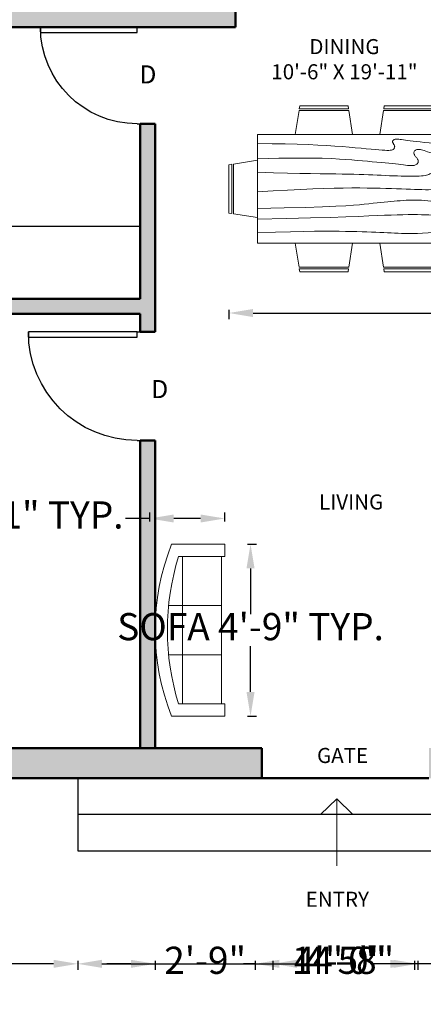
# Model space of a CAD drawing. Units: inches. Extents: x 2568 to 3190, y 746 to 1467.
# Tile 2 of 7: x 2767 to 2900, y 746 to 1073. Entities that reach past the tile are written whole.
import ezdxf

# ---------------------------------------------------------------- set-up
doc = ezdxf.new("R2010")
doc.units = ezdxf.units.IN
for name, color, linetype, lineweight in [('A-ANNO-DIMS', 2, 'Continuous', 18), ('A-ANNO-SYMB', 7, 'Continuous', 18), ('A-ANNO-TEXT', 7, 'Continuous', 18), ('A-AREA-IDEN', 7, 'Continuous', 25), ('A-DOOR', 3, 'Continuous', 25), ('A-FLOR-CASE', 8, 'Continuous', 25), ('A-FLOR-STRS', 7, 'Continuous', 25), ('A-FURN', 8, 'Continuous', 18), ('A-WALL', 7, 'Continuous', 50), ('A-WALL-PATT', 252, 'Continuous', 13)]:
    doc.layers.add(name, color=color, linetype=linetype, lineweight=lineweight)
doc.styles.get("Standard").update_dxf_attribs({"font": 'arial.ttf'})
doc.dimstyles.new('ISO-25', dxfattribs={"dimtxt": 9, "dimasz": 8, "dimexe": 2, "dimexo": 1, "dimtad": 0, "dimtih": 1, "dimtoh": 1, "dimdec": 1, "dimlunit": 3, "dimtxsty": 'Standard', "dimcen": 2.5, "dimclrd": 1, "dimclre": 3, "dimclrt": 6, "dimadec": 0, "dimazin": 0, "dimtfac": 1, "dimtdec": 1, "dimtmove": 0, "dimatfit": 3, "dimfxl": 1, "dimfxlon": 1, "dimarcsym": 0})

# ---------------------------------------------------------------- blocks, each defined once
blk = doc.blocks.new('*U7')
for p, q in [((0, 0), (0, -6)), ((36, 0), (36, -6))]:
    blk.add_line(p, q)
blk.add_lwpolyline([(0, 0), (0, 36), (1.75, 36), (1.75, 0)], close=True)
blk.add_arc((0, 0), 36, 0, 90)
blk = doc.blocks.new('*U8')
for p, q in [((0, 0), (0, -6)), ((32, 0), (32, -6))]:
    blk.add_line(p, q)
blk.add_lwpolyline([(0, 0), (0, 32), (1.75, 32), (1.75, 0)], close=True)
blk.add_arc((0, 0), 32, 0, 90)
blk = doc.blocks.new('Dining Set - 36 x 72 in.')
for p, q in [((-22, 27.5), (-22.1562, 26.50042)), ((-5.8416, 26.5), (-22.1534, 26.5)), ((-22, 27.5), (-6, 27.5)), ((-5.8437, 26.49966), (-6, 27.5)), ((6, 27.5), (5.8438, 26.50042)), ((22.1584, 26.5), (5.8466, 26.5)), ((6, 27.5), (22, 27.5)), ((22.1563, 26.49966), (22, 27.5)), ((-22.2343, 26.00059), (-23.4847, 17.99762)), ((-22.2304, 26), (-5.7608, 26)), ((-4.5152, 17.99762), (-5.7655, 25.99926)), ((5.7657, 26.00059), (4.5153, 17.99762)), ((5.7696, 26), (22.2392, 26)), ((23.4848, 17.99762), (22.2345, 25.99926)), ((36, 18), (-36, 18)), ((-36, 18), (-36, -18)), ((36, -18), (36, 18)), ((-45.5, 8), (-44.5004, 8.15617)), ((-45.5, 8), (-45.5, -8)), ((-44.5, -8.15843), (-44.5, 8.15338)), ((-44.0006, 8.23428), (-35.9976, 9.48474)), ((-44, 8.23041), (-44, -8.23915)), ((44.0006, 8.23428), (35.9976, 9.48474)), ((44, 8.23041), (44, -8.23915)), ((44.5, -8.15843), (44.5, 8.15338)), ((45.5, 8), (44.5005, 8.15617)), ((45.5, 8), (45.5, -8)), ((-44.4997, -8.15631), (-45.5, -8)), ((-35.9976, -9.48476), (-43.9993, -8.2345)), ((35.9976, -9.48476), (43.9993, -8.2345)), ((44.4997, -8.15631), (45.5, -8)), ((-36, -18), (36, -18)), ((-22.2343, -26.0006), (-23.4847, -17.99762)), ((-4.5152, -17.99762), (-5.7655, -25.99928)), ((5.7657, -26.0006), (4.5153, -17.99762)), ((23.4848, -17.99762), (22.2345, -25.99928)), ((-22.2304, -26), (-5.7608, -26)), ((5.7696, -26), (22.2392, -26)), ((-22, -27.5), (-22.1562, -26.50044)), ((-5.8416, -26.5), (-22.1534, -26.5)), ((-22, -27.5), (-6, -27.5)), ((-5.8437, -26.49967), (-6, -27.5)), ((6, -27.5), (5.8438, -26.50044)), ((22.1584, -26.5), (5.8466, -26.5)), ((6, -27.5), (22, -27.5)), ((22.1563, -26.49967), (22, -27.5))]:
    blk.add_line(p, q)
for points in [[(-36, 15), (-31.1772, 14.97754), (-26.8079, 14.91406), (-22.8538, 14.81543), (-19.276, 14.6875), (-16.0362, 14.53613), (-13.0957, 14.36718), (-10.4159, 14.18652), (-7.9583, 14), (-5.6904, 13.81315), (-3.6035, 13.63021), (-1.6954, 13.45508), (0.0365, 13.29166), (1.5945, 13.14388), (2.9811, 13.01562), (4.1988, 12.9108), (5.25, 12.83333), (6.1393, 12.78613), (6.8802, 12.76823), (7.4883, 12.77767), (7.9792, 12.8125), (8.3685, 12.87077), (8.6719, 12.95052), (8.9049, 13.0498), (9.0833, 13.16666), (9.2205, 13.29899), (9.3216, 13.44401), (9.3895, 13.59879), (9.4271, 13.76041), (9.4373, 13.92594), (9.4232, 14.09245), (9.3875, 14.257), (9.3333, 14.41666), (9.2638, 14.56917), (9.1836, 14.71484), (9.0975, 14.85465), (9.0104, 14.98958), (8.9272, 15.1206), (8.8529, 15.2487), (8.7922, 15.37483), (8.75, 15.5), (8.7305, 15.62467), (8.7344, 15.74739), (8.7617, 15.86621), (8.8125, 15.97916), (8.8867, 16.08431), (8.9844, 16.17968), (9.1055, 16.26334), (9.25, 16.33333), (9.4189, 16.38802), (9.6172, 16.42708), (9.8506, 16.45052), (10.125, 16.45833), (10.4463, 16.45052), (10.8203, 16.42708), (11.2529, 16.38802), (11.75, 16.33333), (12.3184, 16.26318), (12.9694, 16.17838), (13.7151, 16.07991), (14.5677, 15.96875), (15.5395, 15.84586), (16.6426, 15.71224), (17.8893, 15.56884), (19.2917, 15.41666), (20.859, 15.25667), (22.5879, 15.08984), (24.4721, 14.91715), (26.5052, 14.73958), (28.6809, 14.5581), (30.9929, 14.3737), (33.4347, 14.18733), (36, 14)], [(-36, 10), (-28.9766, 10.14274), (-23.1725, 10.20442), (-18.4241, 10.19775), (-14.5677, 10.13541), (-11.4399, 10.03011), (-8.877, 9.89453), (-6.7154, 9.74137), (-4.7917, 9.58333), (-2.9698, 9.43082), (-1.2246, 9.28515), (0.4415, 9.14534), (2.026, 9.01041), (3.5266, 8.87939), (4.9408, 8.7513), (6.266, 8.62516), (7.5, 8.5), (8.6411, 8.37549), (9.6914, 8.2539), (10.6538, 8.13818), (11.5312, 8.03125), (12.3267, 7.93603), (13.043, 7.85547), (13.6831, 7.79248), (14.25, 7.75), (14.7471, 7.7303), (15.1797, 7.73307), (15.5537, 7.75732), (15.875, 7.80208), (16.1494, 7.86637), (16.3828, 7.94922), (16.5811, 8.04964), (16.75, 8.16666), (16.8944, 8.29915), (17.0143, 8.44531), (17.1089, 8.60319), (17.1771, 8.77083), (17.218, 8.94629), (17.2305, 9.1276), (17.2137, 9.31282), (17.1667, 9.5), (17.0895, 9.6875), (16.987, 9.875), (16.8649, 10.0625), (16.7292, 10.25), (16.5856, 10.4375), (16.4401, 10.625), (16.2985, 10.8125), (16.1667, 11), (16.05, 11.18733), (15.9518, 11.3737), (15.8752, 11.5581), (15.8229, 11.73958), (15.798, 11.91715), (15.8034, 12.08984), (15.842, 12.25667), (15.9167, 12.41666), (16.0295, 12.56836), (16.1784, 12.70833), (16.3605, 12.83268), (16.5729, 12.9375), (16.8127, 13.01888), (17.0768, 13.07291), (17.3625, 13.0957), (17.6667, 13.08333), (17.9894, 13.03312), (18.3418, 12.94726), (18.7382, 12.82918), (19.1927, 12.68229), (19.7195, 12.51001), (20.3327, 12.31575), (21.0465, 12.10294), (21.875, 11.875), (22.8357, 11.63354), (23.959, 11.37304), (25.2786, 11.08618), (26.8282, 10.76562), (28.6414, 10.40405), (30.752, 9.99414), (33.1936, 9.52856), (36, 9)], [(-36, 5.5), (-30.7157, 5.3348), (-26.069, 5.20963), (-21.9946, 5.11767), (-18.4271, 5.05208), (-15.3009, 5.00602), (-12.5508, 4.97265), (-10.1112, 4.94515), (-7.9167, 4.91666), (-5.909, 4.88167), (-4.0586, 4.83984), (-2.3429, 4.79215), (-0.7396, 4.73958), (0.7739, 4.6831), (2.22, 4.6237), (3.6213, 4.56233), (5, 4.5), (6.373, 4.43782), (7.7344, 4.3776), (9.0723, 4.32129), (10.375, 4.27083), (11.6309, 4.22819), (12.8281, 4.19531), (13.9551, 4.17415), (15, 4.16666), (15.954, 4.17448), (16.819, 4.19791), (17.6001, 4.23698), (18.3021, 4.29166), (18.9299, 4.36198), (19.4883, 4.44791), (19.9823, 4.54948), (20.4167, 4.66666), (20.7969, 4.79899), (21.1302, 4.94401), (21.4245, 5.09879), (21.6875, 5.26041), (21.9271, 5.42594), (22.1511, 5.59245), (22.3672, 5.757), (22.5834, 5.91666), (22.8065, 6.06868), (23.0404, 6.21093), (23.2879, 6.34147), (23.5521, 6.45833), (23.8358, 6.55957), (24.142, 6.64323), (24.4735, 6.70735), (24.8334, 6.75), (25.2235, 6.76969), (25.642, 6.76692), (26.0858, 6.74267), (26.5521, 6.69791), (27.0379, 6.63362), (27.5404, 6.55078), (28.0565, 6.45036), (28.5834, 6.33333), (29.1242, 6.19987), (29.7071, 6.04687), (30.3661, 5.87044), (31.1354, 5.66666), (32.0493, 5.43164), (33.142, 5.16146), (34.4475, 4.85221), (36, 4.5)], [(-36, -1), (-30.7915, -0.6591), (-26.0195, -0.38216), (-21.6519, -0.16284), (-17.6563, 0.00521), (-14.0005, 0.12833), (-10.6523, 0.21289), (-7.5796, 0.26522), (-4.75, 0.29166), (-2.134, 0.29793), (0.2878, 0.28711), (2.5317, 0.26163), (4.6146, 0.22396), (6.5529, 0.17651), (8.3633, 0.12174), (10.0623, 0.06209), (11.6667, 0), (13.1899, -0.06201), (14.6341, -0.1211), (15.9982, -0.17432), (17.2813, -0.21875), (18.4823, -0.25147), (19.6003, -0.26953), (20.6343, -0.27002), (21.5834, -0.25), (22.4481, -0.20768), (23.2357, -0.14584), (23.9549, -0.06836), (24.6146, 0.02083), (25.2235, 0.11784), (25.7904, 0.21875), (26.3241, 0.31966), (26.8334, 0.41666), (27.3265, 0.50618), (27.8099, 0.58593), (28.2894, 0.65397), (28.7709, 0.70833), (29.2601, 0.74707), (29.763, 0.76823), (30.2855, 0.76985), (30.8334, 0.75), (31.4088, 0.70784), (31.9994, 0.64713), (32.589, 0.57275), (33.1615, 0.48958), (33.7008, 0.4025), (34.1908, 0.3164), (34.6153, 0.23616), (34.9584, 0.16666), (35.2099, 0.11165), (35.3848, 0.07031), (35.504, 0.04069), (35.5886, 0.02083), (35.6594, 0.00879), (35.7377, 0.0026), (35.8442, 0.00032), (36, 0)], [(-36, -6.5), (-27.1843, -6.31267), (-20.084, -6.1263), (-14.469, -5.9419), (-10.1094, -5.76042), (-6.7752, -5.58285), (-4.2363, -5.41016), (-2.2629, -5.24333), (-0.625, -5.08334), (0.8708, -4.93099), (2.2715, -4.78646), (3.5872, -4.64974), (4.8281, -4.52084), (6.0046, -4.39974), (7.127, -4.28646), (8.2053, -4.18099), (9.25, -4.08334), (10.2705, -3.99382), (11.2734, -3.91407), (12.2647, -3.84603), (13.25, -3.79167), (14.2354, -3.75293), (15.2266, -3.73177), (16.2295, -3.73015), (17.25, -3.75), (18.2912, -3.79248), (19.3451, -3.85547), (20.4009, -3.93604), (21.4479, -4.03125), (22.4754, -4.13819), (23.4727, -4.25391), (24.4289, -4.37549), (25.3334, -4.5), (26.1785, -4.62492), (26.9694, -4.74935), (27.7145, -4.87281), (28.4219, -4.99479), (29.1, -5.11483), (29.7572, -5.23242), (30.4016, -5.34709), (31.0417, -5.45834), (31.6837, -5.56437), (32.3262, -5.65821), (32.9658, -5.73153), (33.599, -5.77604), (34.2224, -5.78345), (34.8327, -5.74545), (35.4264, -5.65373), (36, -5.5)], [(-36, -10), (-26.4022, -9.81299), (-18.4675, -9.62891), (-11.9839, -9.45069), (-6.7396, -9.28125), (-2.5226, -9.12354), (0.8789, -8.98047), (3.6769, -8.85498), (6.0833, -8.75), (8.2767, -8.66765), (10.3021, -8.60677), (12.1712, -8.56543), (13.8958, -8.54167), (15.4876, -8.53353), (16.9583, -8.53907), (18.3197, -8.55632), (19.5834, -8.58334), (20.7616, -8.61841), (21.8685, -8.66081), (22.9188, -8.71004), (23.9271, -8.76563), (24.9081, -8.82707), (25.8763, -8.89388), (26.8465, -8.96558), (27.8334, -9.04167), (28.8474, -9.12118), (29.8828, -9.20117), (30.93, -9.27824), (31.9792, -9.34896), (33.0205, -9.40991), (34.0443, -9.45768), (35.0407, -9.48885), (36, -9.5)], [(-36, -14.5), (-30.0881, -14.33513), (-25.0332, -14.21224), (-20.7312, -14.12647), (-17.0781, -14.07292), (-13.97, -14.04671), (-11.3027, -14.04297), (-8.9724, -14.05681), (-6.875, -14.08334), (-4.9224, -14.11833), (-3.0905, -14.16016), (-1.3709, -14.20785), (0.2448, -14.26042), (1.7647, -14.3169), (3.1973, -14.3763), (4.5507, -14.43767), (5.8333, -14.5), (7.0554, -14.5621), (8.235, -14.62175), (9.3922, -14.67652), (10.5469, -14.72396), (11.7192, -14.76164), (12.929, -14.78711), (14.1965, -14.79794), (15.5417, -14.79167), (16.9933, -14.76424), (18.6152, -14.70508), (20.4804, -14.60197), (22.6615, -14.44271), (25.2312, -14.21509), (28.2624, -13.9069), (31.8277, -13.50594), (36, -13)]]:
    blk.add_lwpolyline(points)
blk = doc.blocks.new('Sofa - Roundback 7 ft.')
for p, q in [((-12.00002, -32.4421), (-12.00003, -6.5971)), ((11.99997, -32.4421), (11.99998, -6.5971)), ((-36.000027, -34), (-36.000027, -11.4696)), ((-35.999844, -13.3819), (35.9998, -13.3819)), ((35.99998, -34), (35.99998, -11.4696)), ((-36.000027, -32.4421), (35.99998, -32.4421))]:
    blk.add_line(p, q)
for points in [[(-36.000027, -34), (-42.000027, -34), (-42.000027, -8)], [(41.99998, -8), (41.99998, -34), (35.99998, -34)]]:
    blk.add_lwpolyline(points)
for centre, radius, start, end in [((0, -114.25), 114.25, 68.43141, 111.5686), ((-0.00001, -127.1968), 121.1968, 72.72033, 107.2797)]:
    blk.add_arc(centre, radius, start, end)
blk = doc.blocks.new('*D25')
at = {"layer": 'A-ANNO-DIMS', "color": 3, "lineweight": -2, "transparency": 16777216}
for p, q in [((2842.13, 898.94), (2845.13, 898.94)), ((2842.13, 841.97), (2845.13, 841.97))]:
    blk.add_line(p, q, dxfattribs=at)
at = {"layer": 'A-ANNO-DIMS', "color": 1, "lineweight": -2, "transparency": 16777216}
for p, q in [((2843.13, 890.94), (2843.13, 875.74)), ((2843.13, 849.97), (2843.13, 865.17))]:
    blk.add_line(p, q, dxfattribs=at)
at = {"layer": 'A-ANNO-DIMS', "color": 1, "transparency": 16777216}
for points in [[(2841.79, 890.94), (2844.46, 890.94), (2843.13, 898.94)], [(2841.79, 849.97), (2844.46, 849.97), (2843.13, 841.97)]]:
    blk.add_solid(points, dxfattribs=at)
at = {"layer": 'Defpoints', "color": 0, "transparency": 16777216}
for p in [(2834.58, 898.94), (2843.13, 898.94), (2834.58, 841.97)]:
    blk.add_point(p, dxfattribs=at)
at = {"layer": 'A-ANNO-DIMS', "color": 6, "transparency": 16777216, "insert": (2843.13, 870.46), "char_height": 9, "attachment_point": 5}
blk.add_mtext('SOFA 4\'-9" TYP.', dxfattribs=at)
blk = doc.blocks.new('*D26')
at = {"layer": 'A-ANNO-DIMS', "color": 1, "lineweight": -2, "transparency": 16777216}
for p, q in [((2809.71, 907.49), (2801.71, 907.49)), ((2826.58, 907.49), (2817.71, 907.49))]:
    blk.add_line(p, q, dxfattribs=at)
at = {"layer": 'A-ANNO-DIMS', "color": 3, "lineweight": -2, "transparency": 16777216}
for p, q in [((2809.71, 906.49), (2809.71, 909.49)), ((2834.58, 906.49), (2834.58, 909.49))]:
    blk.add_line(p, q, dxfattribs=at)
at = {"layer": 'A-ANNO-DIMS', "color": 1, "transparency": 16777216}
for points in [[(2817.71, 908.82), (2817.71, 906.15), (2809.71, 907.49)], [(2826.58, 908.82), (2826.58, 906.15), (2834.58, 907.49)]]:
    blk.add_solid(points, dxfattribs=at)
at = {"layer": 'Defpoints', "color": 0, "transparency": 16777216}
for p in [(2809.71, 907.49), (2809.71, 898.94), (2834.58, 898.94)]:
    blk.add_point(p, dxfattribs=at)
at = {"layer": 'A-ANNO-DIMS', "color": 6, "transparency": 16777216, "insert": (2773.58, 907.49), "char_height": 9, "attachment_point": 5}
blk.add_mtext('2\'-1" TYP.', dxfattribs=at)
blk = doc.blocks.new('*D37')
at = {"layer": 'A-ANNO-DIMS', "color": 3, "lineweight": -2, "transparency": 16777216}
for p, q in [((2835.95, 976.61), (2835.95, 973.61)), ((2926.95, 976.61), (2926.95, 973.61))]:
    blk.add_line(p, q, dxfattribs=at)
at = {"layer": 'A-ANNO-DIMS', "color": 1, "lineweight": -2, "transparency": 16777216}
for p, q in [((2843.95, 975.61), (2918.95, 975.61)), ((2926.95, 975.61), (2934.95, 975.61))]:
    blk.add_line(p, q, dxfattribs=at)
at = {"layer": 'A-ANNO-DIMS', "color": 1, "transparency": 16777216}
for points in [[(2843.95, 976.94), (2843.95, 974.27), (2835.95, 975.61)], [(2918.95, 976.94), (2918.95, 974.27), (2926.95, 975.61)]]:
    blk.add_solid(points, dxfattribs=at)
at = {"layer": 'Defpoints', "color": 0, "transparency": 16777216}
for p in [(2835.95, 989.26), (2926.95, 989.26), (2926.95, 975.61)]:
    blk.add_point(p, dxfattribs=at)
at = {"layer": 'A-ANNO-DIMS', "color": 6, "transparency": 16777216, "insert": (2985.04, 975.61), "char_height": 9, "attachment_point": 5}
blk.add_mtext('DINING SET 7\'-7"', dxfattribs=at)
blk = doc.blocks.new('*D41')
at = {"layer": 'A-ANNO-DIMS', "color": 3, "lineweight": -2, "transparency": 16777216}
for p, q in [((2811.52, 760.85), (2811.52, 757.85)), ((2844.66, 760.85), (2844.66, 757.85))]:
    blk.add_line(p, q, dxfattribs=at)
at = {"layer": 'A-ANNO-DIMS', "color": 1, "lineweight": -2, "transparency": 16777216}
for p, q in [((2803.52, 759.85), (2795.52, 759.85)), ((2811.52, 759.85), (2815.43, 759.85)), ((2844.66, 759.85), (2840.76, 759.85)), ((2852.66, 759.85), (2860.66, 759.85))]:
    blk.add_line(p, q, dxfattribs=at)
at = {"layer": 'A-ANNO-DIMS', "color": 1, "transparency": 16777216}
for points in [[(2803.52, 761.18), (2803.52, 758.51), (2811.52, 759.85)], [(2852.66, 761.18), (2852.66, 758.51), (2844.66, 759.85)]]:
    blk.add_solid(points, dxfattribs=at)
at = {"layer": 'Defpoints', "color": 0, "transparency": 16777216}
for p in [(2811.52, 1411.35), (2844.66, 1411.35), (2844.66, 759.85)]:
    blk.add_point(p, dxfattribs=at)
at = {"layer": 'A-ANNO-DIMS', "color": 6, "transparency": 16777216, "insert": (2828.09, 759.85), "char_height": 9, "attachment_point": 5}
blk.add_mtext('2\'-9"', dxfattribs=at)
blk = doc.blocks.new('*D42')
at = {"layer": 'A-ANNO-DIMS', "color": 3, "lineweight": -2, "transparency": 16777216}
for p, q in [((2844.66, 760.85), (2844.66, 757.85)), ((2897.43, 760.85), (2897.43, 757.85))]:
    blk.add_line(p, q, dxfattribs=at)
at = {"layer": 'A-ANNO-DIMS', "color": 1, "lineweight": -2, "transparency": 16777216}
for p, q in [((2852.66, 759.85), (2858.28, 759.85)), ((2889.43, 759.85), (2883.81, 759.85))]:
    blk.add_line(p, q, dxfattribs=at)
at = {"layer": 'A-ANNO-DIMS', "color": 1, "transparency": 16777216}
for points in [[(2852.66, 761.18), (2852.66, 758.51), (2844.66, 759.85)], [(2889.43, 761.18), (2889.43, 758.51), (2897.43, 759.85)]]:
    blk.add_solid(points, dxfattribs=at)
at = {"layer": 'Defpoints', "color": 0, "transparency": 16777216}
for p in [(2844.66, 1411.35), (2897.43, 1411.35), (2897.43, 759.85)]:
    blk.add_point(p, dxfattribs=at)
at = {"layer": 'A-ANNO-DIMS', "color": 6, "transparency": 16777216, "insert": (2871.04, 759.85), "char_height": 9, "attachment_point": 5}
blk.add_mtext('4\'-5"', dxfattribs=at)
blk = doc.blocks.new('*D47')
at = {"layer": 'A-ANNO-DIMS', "color": 3, "lineweight": -2, "transparency": 16777216}
for p, q in [((2754.37, 1452.8), (2754.37, 1455.8)), ((2846.86, 1452.8), (2846.86, 1455.8))]:
    blk.add_line(p, q, dxfattribs=at)
at = {"layer": 'A-ANNO-DIMS', "color": 1, "lineweight": -2, "transparency": 16777216}
for p, q in [((2762.37, 1453.8), (2777.58, 1453.8)), ((2838.86, 1453.8), (2823.65, 1453.8))]:
    blk.add_line(p, q, dxfattribs=at)
at = {"layer": 'A-ANNO-DIMS', "color": 1, "transparency": 16777216}
for points in [[(2762.37, 1455.13), (2762.37, 1452.47), (2754.37, 1453.8)], [(2838.86, 1455.13), (2838.86, 1452.47), (2846.86, 1453.8)]]:
    blk.add_solid(points, dxfattribs=at)
at = {"layer": 'Defpoints', "color": 0, "transparency": 16777216}
for p in [(2846.86, 1453.8), (2754.37, 831.35), (2846.86, 831.35)]:
    blk.add_point(p, dxfattribs=at)
at = {"layer": 'A-ANNO-DIMS', "color": 6, "transparency": 16777216, "insert": (2800.61, 1453.8), "char_height": 9, "attachment_point": 5}
blk.add_mtext('7\'-8 1/2"', dxfattribs=at)
blk = doc.blocks.new('*D50')
at = {"layer": 'A-ANNO-DIMS', "color": 1, "lineweight": -2, "transparency": 16777216}
for p, q in [((2838.86, 1453.8), (2830.86, 1453.8)), ((2846.86, 1453.8), (2851.29, 1453.8)), ((2902.21, 1453.8), (2897.79, 1453.8)), ((2910.21, 1453.8), (2918.21, 1453.8))]:
    blk.add_line(p, q, dxfattribs=at)
at = {"layer": 'A-ANNO-DIMS', "color": 3, "lineweight": -2, "transparency": 16777216}
for p, q in [((2846.86, 1452.8), (2846.86, 1455.8)), ((2902.21, 1452.8), (2902.21, 1455.8))]:
    blk.add_line(p, q, dxfattribs=at)
at = {"layer": 'A-ANNO-DIMS', "color": 1, "transparency": 16777216}
for points in [[(2838.86, 1455.13), (2838.86, 1452.47), (2846.86, 1453.8)], [(2910.21, 1455.13), (2910.21, 1452.47), (2902.21, 1453.8)]]:
    blk.add_solid(points, dxfattribs=at)
at = {"layer": 'Defpoints', "color": 0, "transparency": 16777216}
for p in [(2902.21, 1453.8), (2846.86, 831.35), (2902.21, 831.35)]:
    blk.add_point(p, dxfattribs=at)
at = {"layer": 'A-ANNO-DIMS', "color": 6, "transparency": 16777216, "insert": (2874.54, 1453.8), "char_height": 9, "attachment_point": 5}
blk.add_mtext('4\'-7 1/2"', dxfattribs=at)
blk = doc.blocks.new('*D51')
at = {"layer": 'A-ANNO-DIMS', "color": 3, "lineweight": -2, "transparency": 16777216}
for p, q in [((2785.87, 760.85), (2785.87, 757.85)), ((2961.66, 760.85), (2961.66, 757.85))]:
    blk.add_line(p, q, dxfattribs=at)
at = {"layer": 'A-ANNO-DIMS', "color": 1, "lineweight": -2, "transparency": 16777216}
for p, q in [((2793.87, 759.85), (2858.1, 759.85)), ((2953.66, 759.85), (2889.42, 759.85))]:
    blk.add_line(p, q, dxfattribs=at)
at = {"layer": 'A-ANNO-DIMS', "color": 1, "transparency": 16777216}
for points in [[(2793.87, 761.18), (2793.87, 758.51), (2785.87, 759.85)], [(2953.66, 761.18), (2953.66, 758.51), (2961.66, 759.85)]]:
    blk.add_solid(points, dxfattribs=at)
at = {"layer": 'Defpoints', "color": 0, "transparency": 16777216}
for p in [(2785.87, 797.35), (2961.66, 797.35), (2961.66, 759.85)]:
    blk.add_point(p, dxfattribs=at)
at = {"layer": 'A-ANNO-DIMS', "color": 6, "transparency": 16777216, "insert": (2873.76, 759.85), "char_height": 9, "attachment_point": 5}
blk.add_mtext('14\'-8"', dxfattribs=at)
blk = doc.blocks.new('*D52')
at = {"layer": 'A-ANNO-DIMS', "color": 1, "lineweight": -2, "transparency": 16777216}
for p, q in [((2602.07, 821.35), (2602.07, 829.35)), ((2602.07, 829.35), (2610.07, 829.35)), ((2602.07, 805.35), (2602.07, 813.35))]:
    blk.add_line(p, q, dxfattribs=at)
at = {"layer": 'A-ANNO-DIMS', "color": 3, "lineweight": -2, "transparency": 16777216}
for p, q in [((2603.07, 821.35), (2600.07, 821.35)), ((2603.07, 797.35), (2600.07, 797.35))]:
    blk.add_line(p, q, dxfattribs=at)
at = {"layer": 'A-ANNO-DIMS', "color": 1, "transparency": 16777216}
for points in [[(2600.74, 813.35), (2603.41, 813.35), (2602.07, 821.35)], [(2600.74, 805.35), (2603.41, 805.35), (2602.07, 797.35)]]:
    blk.add_solid(points, dxfattribs=at)
at = {"layer": 'Defpoints', "color": 0, "transparency": 16777216}
for p in [(2602.07, 821.35), (2785.87, 821.35), (2785.87, 797.35)]:
    blk.add_point(p, dxfattribs=at)
at = {"layer": 'A-ANNO-DIMS', "color": 6, "transparency": 16777216, "insert": (2622.74, 829.35), "char_height": 9, "attachment_point": 5}
blk.add_mtext('2\'-0"', dxfattribs=at)
blk = doc.blocks.new('*D54')
at = {"layer": 'A-ANNO-DIMS', "color": 3, "lineweight": -2, "transparency": 16777216}
for p, q in [((2850.52, 760.85), (2850.52, 757.85)), ((2898.52, 760.85), (2898.52, 757.85))]:
    blk.add_line(p, q, dxfattribs=at)
at = {"layer": 'A-ANNO-DIMS', "color": 1, "lineweight": -2, "transparency": 16777216}
for p, q in [((2858.52, 759.85), (2861.75, 759.85)), ((2890.52, 759.85), (2887.29, 759.85))]:
    blk.add_line(p, q, dxfattribs=at)
at = {"layer": 'A-ANNO-DIMS', "color": 1, "transparency": 16777216}
for points in [[(2858.52, 761.18), (2858.52, 758.51), (2850.52, 759.85)], [(2890.52, 761.18), (2890.52, 758.51), (2898.52, 759.85)]]:
    blk.add_solid(points, dxfattribs=at)
at = {"layer": 'Defpoints', "color": 0, "transparency": 16777216}
for p in [(2850.52, 1310.35), (2898.52, 1310.35), (2898.52, 759.85)]:
    blk.add_point(p, dxfattribs=at)
at = {"layer": 'A-ANNO-DIMS', "color": 6, "transparency": 16777216, "insert": (2874.52, 759.85), "char_height": 9, "attachment_point": 5}
blk.add_mtext('4\'-0"', dxfattribs=at)
blk = doc.blocks.new('*D56')
at = {"layer": 'A-ANNO-DIMS', "color": 3, "lineweight": -2, "transparency": 16777216}
for p, q in [((2603.07, 1070.35), (2600.07, 1070.35)), ((2603.07, 1034.35), (2600.07, 1034.35))]:
    blk.add_line(p, q, dxfattribs=at)
at = {"layer": 'A-ANNO-DIMS', "color": 1, "lineweight": -2, "transparency": 16777216}
for p, q in [((2602.07, 1062.35), (2602.07, 1057.57)), ((2602.07, 1042.35), (2602.07, 1047.13))]:
    blk.add_line(p, q, dxfattribs=at)
at = {"layer": 'A-ANNO-DIMS', "color": 1, "transparency": 16777216}
for points in [[(2600.74, 1062.35), (2603.41, 1062.35), (2602.07, 1070.35)], [(2600.74, 1042.35), (2603.41, 1042.35), (2602.07, 1034.35)]]:
    blk.add_solid(points, dxfattribs=at)
at = {"layer": 'Defpoints', "color": 0, "transparency": 16777216}
for p in [(2602.07, 1070.35), (2974.52, 1070.35), (2974.52, 1034.35)]:
    blk.add_point(p, dxfattribs=at)
at = {"layer": 'A-ANNO-DIMS', "color": 6, "transparency": 16777216, "insert": (2602.07, 1052.35), "char_height": 9, "attachment_point": 5}
blk.add_mtext('3\'-0"', dxfattribs=at)
blk = doc.blocks.new('*D58')
at = {"layer": 'A-ANNO-DIMS', "color": 3, "lineweight": -2, "transparency": 16777216}
for p, q in [((2603.07, 1029.35), (2600.07, 1029.35)), ((2603.07, 980.35), (2600.07, 980.35))]:
    blk.add_line(p, q, dxfattribs=at)
at = {"layer": 'A-ANNO-DIMS', "color": 1, "lineweight": -2, "transparency": 16777216}
for p, q in [((2602.07, 1021.35), (2602.07, 1009.99)), ((2602.07, 988.35), (2602.07, 999.71))]:
    blk.add_line(p, q, dxfattribs=at)
at = {"layer": 'A-ANNO-DIMS', "color": 1, "transparency": 16777216}
for points in [[(2600.74, 1021.35), (2603.41, 1021.35), (2602.07, 1029.35)], [(2600.74, 988.35), (2603.41, 988.35), (2602.07, 980.35)]]:
    blk.add_solid(points, dxfattribs=at)
at = {"layer": 'Defpoints', "color": 0, "transparency": 16777216}
for p in [(3044.52, 1029.35), (2602.07, 980.35), (3043.77, 980.35)]:
    blk.add_point(p, dxfattribs=at)
at = {"layer": 'A-ANNO-DIMS', "color": 6, "transparency": 16777216, "insert": (2602.07, 1004.85), "char_height": 9, "attachment_point": 5}
blk.add_mtext('4\'-1"', dxfattribs=at)
blk = doc.blocks.new('*D62')
at = {"layer": 'A-ANNO-DIMS', "color": 3, "lineweight": -2, "transparency": 16777216}
for p, q in [((2603.07, 1004.35), (2600.07, 1004.35)), ((2603.07, 980.35), (2600.07, 980.35))]:
    blk.add_line(p, q, dxfattribs=at)
at = {"layer": 'A-ANNO-DIMS', "color": 1, "lineweight": -2, "transparency": 16777216}
for p, q in [((2602.07, 996.35), (2602.07, 988.35)), ((2602.07, 980.35), (2602.07, 972.35)), ((2602.07, 972.35), (2594.07, 972.35))]:
    blk.add_line(p, q, dxfattribs=at)
at = {"layer": 'A-ANNO-DIMS', "color": 1, "transparency": 16777216}
for points in [[(2600.74, 996.35), (2603.41, 996.35), (2602.07, 1004.35)], [(2600.74, 988.35), (2603.41, 988.35), (2602.07, 980.35)]]:
    blk.add_solid(points, dxfattribs=at)
at = {"layer": 'Defpoints', "color": 0, "transparency": 16777216}
for p in [(3044.52, 1004.35), (2602.07, 980.35), (3043.77, 980.35)]:
    blk.add_point(p, dxfattribs=at)
at = {"layer": 'A-ANNO-DIMS', "color": 6, "transparency": 16777216, "insert": (2581.41, 972.35), "char_height": 9, "attachment_point": 5}
blk.add_mtext('2\'-0"', dxfattribs=at)
blk = doc.blocks.new('*D63')
at = {"layer": 'A-ANNO-DIMS', "color": 1, "lineweight": -2, "transparency": 16777216}
for p, q in [((3146.97, 1004.35), (3146.97, 1012.35)), ((3146.97, 1012.35), (3154.97, 1012.35)), ((3146.97, 988.35), (3146.97, 996.35))]:
    blk.add_line(p, q, dxfattribs=at)
at = {"layer": 'A-ANNO-DIMS', "color": 3, "lineweight": -2, "transparency": 16777216}
for p, q in [((3145.97, 1004.35), (3148.97, 1004.35)), ((3145.97, 980.35), (3148.97, 980.35))]:
    blk.add_line(p, q, dxfattribs=at)
at = {"layer": 'A-ANNO-DIMS', "color": 1, "transparency": 16777216}
for points in [[(3145.64, 996.35), (3148.31, 996.35), (3146.97, 1004.35)], [(3145.64, 988.35), (3148.31, 988.35), (3146.97, 980.35)]]:
    blk.add_solid(points, dxfattribs=at)
at = {"layer": 'Defpoints', "color": 0, "transparency": 16777216}
for p in [(2806.52, 1004.35), (3146.97, 1004.35), (2806.52, 980.35)]:
    blk.add_point(p, dxfattribs=at)
at = {"layer": 'A-ANNO-DIMS', "color": 6, "transparency": 16777216, "insert": (3167.64, 1012.35), "char_height": 9, "attachment_point": 5}
blk.add_mtext('2\'-0"', dxfattribs=at)
blk = doc.blocks.new('*D74')
at = {"layer": 'A-ANNO-DIMS', "color": 3, "lineweight": -2, "transparency": 16777216}
for p, q in [((2603.07, 1070.35), (2600.07, 1070.35)), ((2603.07, 1038.35), (2600.07, 1038.35))]:
    blk.add_line(p, q, dxfattribs=at)
at = {"layer": 'A-ANNO-DIMS', "color": 1, "lineweight": -2, "transparency": 16777216}
for p, q in [((2602.07, 1062.35), (2602.07, 1059.57)), ((2602.07, 1046.35), (2602.07, 1049.13))]:
    blk.add_line(p, q, dxfattribs=at)
at = {"layer": 'A-ANNO-DIMS', "color": 1, "transparency": 16777216}
for points in [[(2600.74, 1062.35), (2603.41, 1062.35), (2602.07, 1070.35)], [(2600.74, 1046.35), (2603.41, 1046.35), (2602.07, 1038.35)]]:
    blk.add_solid(points, dxfattribs=at)
at = {"layer": 'Defpoints', "color": 0, "transparency": 16777216}
for p in [(2602.07, 1070.35), (2806.52, 1070.35), (2806.52, 1038.35)]:
    blk.add_point(p, dxfattribs=at)
at = {"layer": 'A-ANNO-DIMS', "color": 6, "transparency": 16777216, "insert": (2602.07, 1054.35), "char_height": 9, "attachment_point": 5}
blk.add_mtext('2\'-8"', dxfattribs=at)
blk = doc.blocks.new('*D83')
at = {"layer": 'A-ANNO-DIMS', "color": 3, "lineweight": -2, "transparency": 16777216}
for p, q in [((2754.37, 760.85), (2754.37, 757.85)), ((2785.87, 760.85), (2785.87, 757.85))]:
    blk.add_line(p, q, dxfattribs=at)
at = {"layer": 'A-ANNO-DIMS', "color": 1, "lineweight": -2, "transparency": 16777216}
for p, q in [((2754.37, 759.85), (2746.37, 759.85)), ((2777.87, 759.85), (2762.37, 759.85))]:
    blk.add_line(p, q, dxfattribs=at)
at = {"layer": 'A-ANNO-DIMS', "color": 1, "transparency": 16777216}
for points in [[(2762.37, 761.18), (2762.37, 758.51), (2754.37, 759.85)], [(2777.87, 761.18), (2777.87, 758.51), (2785.87, 759.85)]]:
    blk.add_solid(points, dxfattribs=at)
at = {"layer": 'Defpoints', "color": 0, "transparency": 16777216}
for p in [(2754.37, 821.35), (2785.87, 797.35), (2754.37, 759.85)]:
    blk.add_point(p, dxfattribs=at)
at = {"layer": 'A-ANNO-DIMS', "color": 6, "transparency": 16777216, "insert": (2723.22, 759.85), "char_height": 9, "attachment_point": 5}
blk.add_mtext('2\'-7 1/2"', dxfattribs=at)

msp = doc.modelspace()

# ---------------------------------------------------------------- hatches: boundary and pattern name
at = {"layer": 'A-WALL-PATT'}
h = msp.add_hatch(color=256, dxfattribs=at)
h.dxf.hatch_style = 1
h.paths.add_polyline_path([(2709.74, 1411.35), (2709.74, 1421.35), (2634.52, 1421.35), (2634.52, 1371.08), (2644.52, 1371.08), (2644.52, 1411.35)])
h.paths.add_polyline_path([(2844.66, 1411.35), (2844.66, 1421.35), (2763.78, 1421.35), (2763.78, 1411.35)])
h.paths.add_polyline_path([(2996.2, 1411.35), (2996.2, 1421.35), (2897.43, 1421.35), (2897.43, 1411.35)])
h.paths.add_polyline_path([(3104.52, 1411.35), (3104.52, 1371.08), (3114.52, 1371.08), (3114.52, 1421.35), (3052.64, 1421.35), (3052.64, 1411.35)])
h.paths.add_polyline_path([(3114.52, 1316.62), (3104.52, 1316.62), (3104.52, 1248.37), (3114.52, 1248.37)])
h.paths.add_polyline_path([(3104.52, 1174.04), (3114.52, 1174.04), (3114.52, 1222.08), (3104.52, 1222.08)])
h.paths.add_polyline_path([(3104.52, 1020.11), (3114.52, 1020.11), (3114.52, 1113), (3104.52, 1113)])
h.paths.add_polyline_path([(3104.52, 920.42), (3114.52, 920.42), (3114.52, 992.96), (3104.52, 992.96)])
h.paths.add_polyline_path([(3114.52, 821.35), (3114.52, 865.93), (3104.52, 865.93), (3104.52, 831.35), (3055.78, 831.35), (3055.78, 821.35)])
h.paths.add_polyline_path([(2902.21, 831.35), (2902.21, 821.35), (2986.63, 821.35), (2986.63, 831.35)])
h.paths.add_polyline_path([(2634.52, 821.35), (2676.76, 821.35), (2676.76, 831.35), (2644.52, 831.35), (2644.52, 865.93), (2634.52, 865.93)])
h.paths.add_polyline_path([(2754.37, 821.35), (2846.86, 821.35), (2846.86, 831.35), (2754.37, 831.35)])
h.paths.add_polyline_path([(2644.52, 920.42), (2644.52, 1002.57), (2634.52, 1002.57), (2634.52, 920.42)])
h.paths.add_polyline_path([(2644.52, 1044.16), (2644.52, 1113), (2634.52, 1113), (2634.52, 1044.16)])
h.paths.add_polyline_path([(2644.52, 1248.37), (2644.52, 1316.62), (2634.52, 1316.62), (2634.52, 1248.37)])
h.paths.add_polyline_path([(2634.52, 1222.08), (2634.52, 1174.04), (2644.52, 1174.04), (2644.52, 1222.08)])
h = msp.add_hatch(color=256, dxfattribs=at)
h.dxf.hatch_style = 1
h.paths.add_polyline_path([(2811.52, 1411.35), (2806.52, 1411.35), (2806.52, 1303.35), (2811.52, 1303.35), (2811.52, 1310.35), (2850.52, 1310.35), (2850.52, 1315.35), (2811.52, 1315.35)])
h.paths.add_polyline_path([(2942.52, 1411.35), (2937.52, 1411.35), (2937.52, 1315.35), (2898.52, 1315.35), (2898.52, 1310.35), (2937.52, 1310.35), (2937.52, 1303.35), (2942.52, 1303.35)])
h.paths.add_polyline_path([(2811.52, 1267.35), (2704.52, 1267.35), (2704.52, 1261.35), (2704.52, 1237.35), (2704.52, 1202.35), (2644.52, 1202.35), (2644.52, 1197.35), (2806.52, 1197.35), (2806.52, 1191.38), (2811.52, 1191.38), (2811.52, 1202.35), (2793.52, 1202.35), (2793.52, 1232.35), (2788.52, 1232.35), (2788.52, 1202.35), (2709.52, 1202.35), (2709.52, 1262.35), (2788.52, 1262.35), (2788.52, 1256.35), (2793.52, 1256.35), (2793.52, 1262.35), (2811.52, 1262.35)])
h.paths.add_polyline_path([(2680.52, 1267.35), (2644.52, 1267.35), (2644.52, 1261.35), (2680.52, 1261.35)])
h.paths.add_polyline_path([(3044.52, 1267.35), (2937.52, 1267.35), (2937.52, 1262.35), (2955.52, 1262.35), (2955.52, 1256.35), (2960.52, 1256.35), (2960.52, 1262.35), (3039.52, 1262.35), (3039.52, 1202.35), (2960.52, 1202.35), (2960.52, 1232.35), (2955.52, 1232.35), (2955.52, 1202.35), (2937.52, 1202.35), (2937.52, 1191.38), (2942.52, 1191.38), (2942.52, 1197.35), (3104.52, 1197.35), (3104.52, 1202.35), (3044.52, 1202.35)])
h.paths.add_polyline_path([(3104.52, 1267.35), (3072.52, 1267.35), (3072.52, 1262.35), (3104.52, 1262.35)])
h.paths.add_polyline_path([(2838.1, 1075.35), (2811.52, 1075.35), (2811.52, 1155.35), (2806.52, 1155.35), (2806.52, 1075.35), (2644.52, 1075.35), (2644.52, 1070.35), (2806.52, 1070.35), (2811.52, 1070.35), (2838.1, 1070.35)])
h.paths.add_polyline_path([(3104.52, 1075.35), (2942.52, 1075.35), (2942.52, 1155.38), (2937.52, 1155.38), (2937.52, 1075.35), (2910.92, 1075.35), (2910.92, 1070.35), (2937.52, 1070.35), (3104.52, 1070.35)])
h.paths.add_polyline_path([(2811.52, 1038.35), (2806.52, 1038.35), (2806.52, 980.35), (2644.52, 980.35), (2644.52, 975.35), (2806.52, 975.35), (2806.52, 969.37), (2811.52, 969.37), (2811.52, 975.35)])
h.paths.add_polyline_path([(3104.52, 980.35), (2937.52, 980.35), (2937.52, 969.35), (2942.52, 969.35), (2942.52, 975.35), (3104.52, 975.35)])
h.paths.add_polyline_path([(3104.52, 1034.35), (3039.52, 1034.35), (3039.52, 1004.35), (3044.52, 1004.35), (3044.52, 1029.35), (3104.52, 1029.35)])
h.paths.add_polyline_path([(2942.52, 933.35), (2937.52, 933.35), (2937.52, 831.35), (2942.52, 831.35)])
h.paths.add_polyline_path([(2811.52, 933.37), (2806.52, 933.37), (2806.52, 831.35), (2811.52, 831.35)])

# ---------------------------------------------------------------- linework, layer by layer
at = {"layer": 'A-ANNO-SYMB'}
for p, q in [((2871.69, 814.57), (2866.33, 809.35)), ((2871.69, 792.3), (2871.69, 814.57)), ((2871.69, 814.57), (2877.05, 809.35))]:
    msp.add_line(p, q, dxfattribs=at)
at = {"layer": 'A-FLOR-CASE'}
msp.add_line((2668.52, 1004.35), (2806.52, 1004.35), dxfattribs=at)
at = {"layer": 'A-FLOR-STRS'}
for p, q in [((2785.87, 821.35), (2785.87, 797.35)), ((2961.66, 809.35), (2785.87, 809.35)), ((2785.87, 797.35), (2961.66, 797.35))]:
    msp.add_line(p, q, dxfattribs=at)
at = {"layer": 'A-WALL'}
for p, q in [((2838.1, 1075.35), (2838.1, 1070.35)), ((2806.52, 1070.35), (2644.52, 1070.35)), ((2806.52, 1070.35), (2838.1, 1070.35)), ((2806.52, 1038.35), (2806.52, 980.35)), ((2806.52, 1038.35), (2811.52, 1038.35)), ((2811.52, 1038.35), (2811.52, 975.35)), ((2806.52, 980.35), (2644.52, 980.35)), ((2806.52, 975.35), (2644.52, 975.35)), ((2806.52, 975.35), (2806.52, 969.37)), ((2811.52, 975.35), (2811.52, 969.37)), ((2811.52, 969.37), (2806.52, 969.37)), ((2811.52, 933.37), (2806.52, 933.37)), ((2806.52, 933.37), (2806.52, 831.35)), ((2811.52, 933.37), (2811.52, 831.35)), ((2644.52, 831.35), (2846.86, 831.35)), ((2846.86, 831.35), (2846.86, 821.35)), ((2634.52, 821.35), (2902.21, 821.35))]:
    msp.add_line(p, q, dxfattribs=at)

# ---------------------------------------------------------------- block references
at = {"layer": 'A-DOOR', "xscale": -1, "rotation": 90}
for name, p in [('*U8', (2805.52, 1070.35)), ('*U7', (2805.52, 969.35))]:
    msp.add_blockref(name, p, dxfattribs=at)
at = {"layer": 'A-FURN'}
msp.add_blockref('Dining Set - 36 x 72 in.', (2881.45, 1016.76), dxfattribs=at)
at = {"layer": 'A-FURN', "xscale": 0.6782133153273913, "yscale": 0.6782133153273913, "zscale": 0.6782133153273913, "rotation": 90}
msp.add_blockref('Sofa - Roundback 7 ft.', (2811.52, 870.46), dxfattribs=at)

# ---------------------------------------------------------------- texts
at = {"layer": 'A-ANNO-TEXT', "attachment_point": 1}
for s, width, insert, char_height in [('D', 7.7602, (2806.31, 1057.71), 6), ('D', 7.7602, (2810.22, 953.38), 6), ('\\pxqc;GATE', 33.0926, (2857.08, 831.42), 5), ('\\pxqc;ENTRY', 69.8646, (2836.95, 783.75), 5)]:
    msp.add_mtext_dynamic_manual_height_columns(s, width=width, gutter_width=12.5, heights=[0], dxfattribs=dict(at, insert=insert, char_height=char_height))
at = {"layer": 'A-AREA-IDEN', "char_height": 5, "attachment_point": 1}
for s, insert in [('\\pxqc;DINING\\P10\'-6" X 19\'-11"', (2839.3, 1066.42)), ('\\pxqc;LIVING', (2841.53, 915.46))]:
    msp.add_mtext_dynamic_manual_height_columns(s, width=69.8646, gutter_width=12.5, heights=[0], dxfattribs=dict(at, insert=insert))

# ---------------------------------------------------------------- dimensions: what is measured, and where the dimension line sits
at = {"layer": 'A-ANNO-DIMS'}
for base, p1, p2, picture, middle in [((2846.86, 1453.8), (2754.37, 831.35), (2846.86, 831.35), '*D47', (2800.61, 1453.8)), ((2902.2147, 1453.7989), (2846.8636, 831.3489), (2902.2147, 831.3489), '*D50', (2874.5391, 1453.7989)), ((2844.66, 759.85), (2811.52, 1411.35), (2844.66, 1411.35), '*D41', (2828.09, 759.85)), ((2897.43, 759.85), (2844.66, 1411.35), (2897.43, 1411.35), '*D42', (2871.04, 759.85)), ((2898.52, 759.85), (2850.52, 1310.35), (2898.52, 1310.35), '*D54', (2874.52, 759.85)), ((2754.37, 759.85), (2785.87, 797.35), (2754.37, 821.35), '*D83', (2723.22, 759.85)), ((2961.66, 759.85), (2785.87, 797.35), (2961.66, 797.35), '*D51', (2873.76, 759.85))]:
    dim = msp.add_linear_dim(base=base, p1=p1, p2=p2, dimstyle='ISO-25', override={"dimdec": 1, "dimlfac": 1, "dimrnd": 0, "dimzin": 1, "dimdsep": 46, "dimlunit": 4, "dimfrac": 2}, dxfattribs=at)
    dim.commit()
    dim.dimension.update_dxf_attribs({"geometry": picture, "text_midpoint": middle})
for base, p1, p2, picture, middle in [((2602.07, 1070.35), (2974.52, 1034.35), (2974.52, 1070.35), '*D56', (2602.07, 1052.35)), ((2602.07, 1070.35), (2806.52, 1038.35), (2806.52, 1070.35), '*D74', (2602.07, 1054.35)), ((2602.07, 980.35), (3044.52, 1029.35), (3043.77, 980.35), '*D58', (2602.07, 1004.85)), ((3146.97, 1004.35), (2806.52, 980.35), (2806.52, 1004.35), '*D63', (3167.64, 1012.35)), ((2602.07, 980.35), (3044.52, 1004.35), (3043.77, 980.35), '*D62', (2581.41, 972.35)), ((2602.07, 821.35), (2785.87, 797.35), (2785.87, 821.35), '*D52', (2622.74, 829.35))]:
    dim = msp.add_linear_dim(base=base, p1=p1, p2=p2, angle=90, dimstyle='ISO-25', override={"dimdec": 1, "dimlfac": 1, "dimrnd": 0, "dimzin": 1, "dimdsep": 46, "dimlunit": 4, "dimfrac": 2}, dxfattribs=at)
    dim.commit()
    dim.dimension.update_dxf_attribs({"geometry": picture, "text_midpoint": middle})
dim = msp.add_linear_dim(base=(2926.95, 975.61), p1=(2835.95, 989.26), p2=(2926.95, 989.26), text='DINING SET <>', dimstyle='ISO-25', override={"dimdec": 1, "dimlfac": 1, "dimrnd": 0, "dimzin": 1, "dimdsep": 46, "dimlunit": 4, "dimfrac": 2}, dxfattribs=at)
dim.commit()
dim.dimension.update_dxf_attribs({"geometry": '*D37', "text_midpoint": (2985.04, 975.61)})
for base, p1, p2, angle, text, picture, middle in [((2809.71, 907.49), (2834.58, 898.94), (2809.71, 898.94), 180, '<> TYP.', '*D26', (2773.58, 907.49)), ((2843.13, 898.94), (2834.58, 841.97), (2834.58, 898.94), 90, 'SOFA <> TYP.', '*D25', (2843.13, 870.46))]:
    dim = msp.add_linear_dim(base=base, p1=p1, p2=p2, angle=angle, text=text, dimstyle='ISO-25', override={"dimdec": 1, "dimlfac": 1, "dimrnd": 0, "dimzin": 1, "dimdsep": 46, "dimlunit": 4, "dimfrac": 2}, dxfattribs=at)
    dim.commit()
    dim.dimension.update_dxf_attribs({"geometry": picture, "text_midpoint": middle})

doc.saveas('drawing.dxf')
